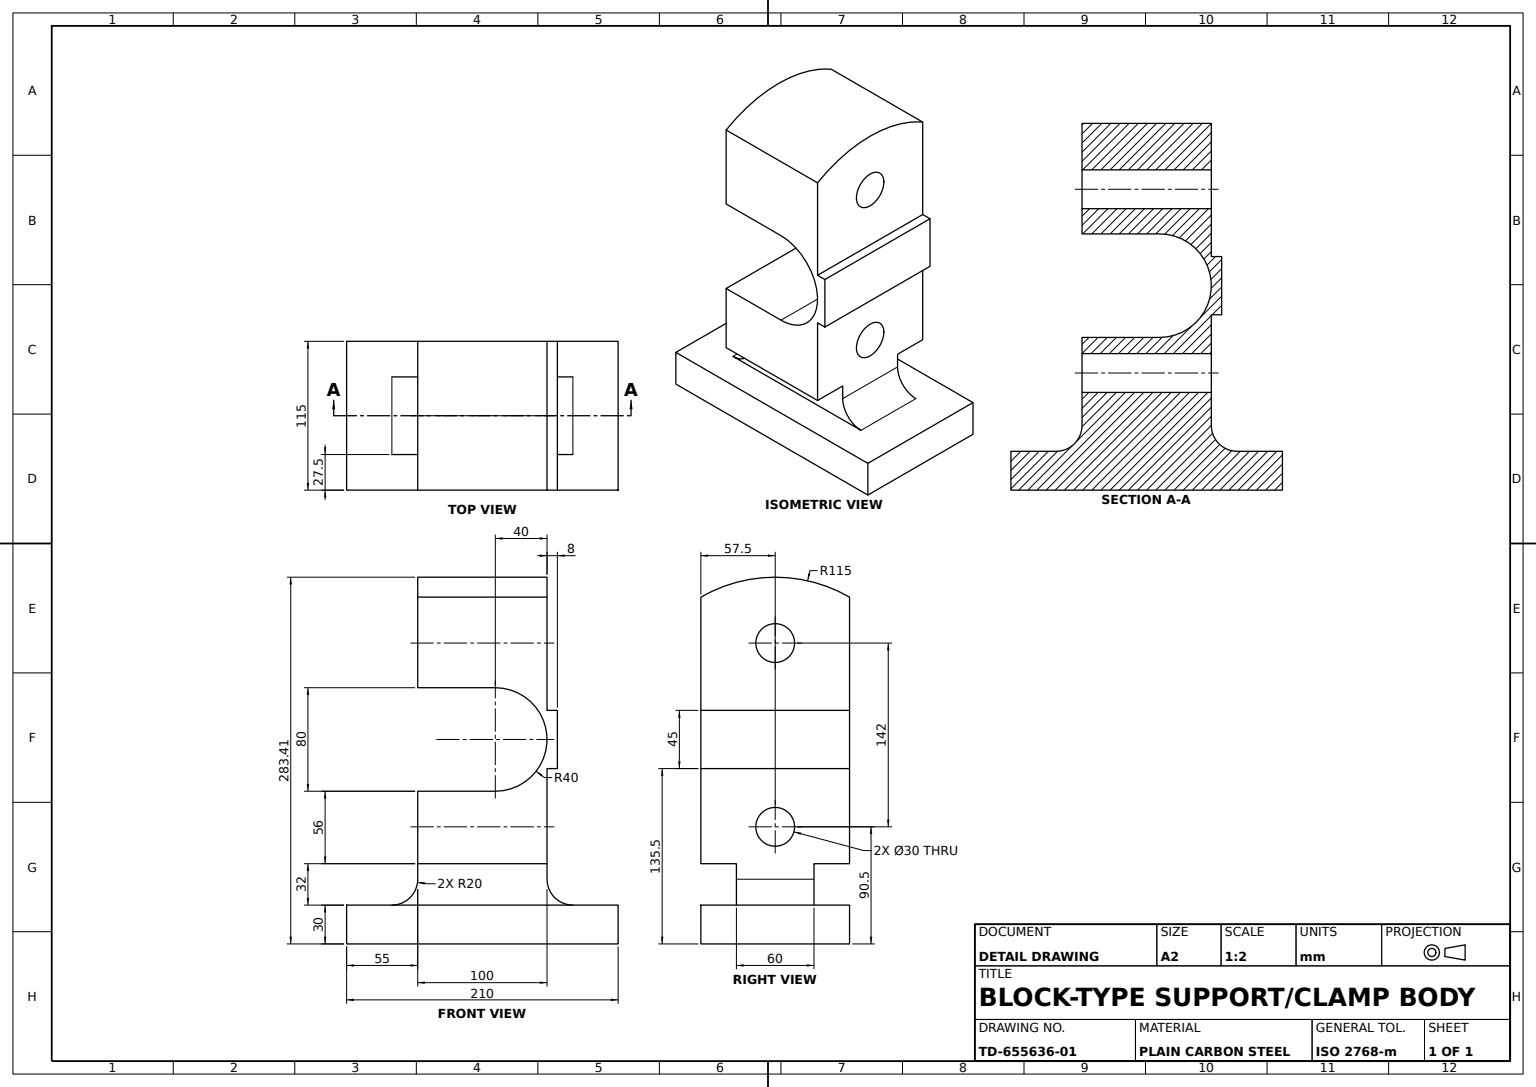
from build123d import *

# Parameters (mm, degrees)
BASE_PLATE_SKETCH_W         = 210
BASE_PLATE_SKETCH_H         = 115
BASE_PLATE_210X115X30_DEPTH = 30
PEDESTAL_SKETCH_W           = 100
PEDESTAL_SKETCH_H           = 60
PEDESTAL_100X60X32_DEPTH    = 32
PEDESTAL_FILLET_R20_R       = 20
CLAMP_BLOCK_DEPTH           = 57.5
CROSS_HOLES_SKETCH_R        = 15
CROSS_HOLES_2X_30_DEPTH     = 115
CLAMP_BAND_DEPTH            = 100


with BuildPart() as part:
    # Base Plate Sketch → Base Plate 210x115x30 (new body)
    with BuildSketch(Plane(origin=(0, 0, 0), x_dir=(1, 0, 0), z_dir=(0, 1, 0))):
        Rectangle(BASE_PLATE_SKETCH_W, BASE_PLATE_SKETCH_H)
    extrude(amount=BASE_PLATE_210X115X30_DEPTH)

    # Pedestal Sketch → Pedestal 100x60x32 (add)
    with BuildSketch(Plane(origin=(0, 30, 0), x_dir=(1, 0, 0), z_dir=(0, 1, 0))):
        Rectangle(PEDESTAL_SKETCH_W, PEDESTAL_SKETCH_H)
    extrude(amount=PEDESTAL_100X60X32_DEPTH)

    # Pedestal Fillet R20
    pedestal_fillet_r20_edges = [part.edges().sort_by_distance(p)[0] for p in [
        (50, 30, 0),
        (-50, 30, 0),
    ]]
    fillet(pedestal_fillet_r20_edges, radius=PEDESTAL_FILLET_R20_R)

    # Clamp Block Profile Sketch → Clamp Block (add, symmetric)
    with BuildSketch(Plane.XY):
        with BuildLine():
            Line((50, 62), (50, 118))
            Line((50, 118), (50, 135.5))
            Line((50, 135.5), (58, 135.5))
            Line((58, 135.5), (58, 180.5))
            Line((58, 180.5), (50, 180.5))
            Line((50, 180.5), (50, 198))
            Line((50, 198), (50, 268))
            Line((50, 268), (-50, 268))
            Line((-50, 268), (-50, 198))
            Line((-50, 198), (10, 198))
            ThreePointArc((10, 198), (50, 158), (10, 118))
            Line((10, 118), (-50, 118))
            Line((-50, 118), (-50, 62))
            Line((-50, 62), (50, 62))
        make_face()
    extrude(amount=CLAMP_BLOCK_DEPTH, both=True)

    # Cross Holes Sketch → Cross Holes 2xØ30 (cut)
    with BuildSketch(Plane.ZY.offset(50)):
        with Locations((0, 90.5)):
            Circle(CROSS_HOLES_SKETCH_R)
        with Locations((0, 232.5)):
            Circle(CROSS_HOLES_SKETCH_R)
    extrude(amount=-CROSS_HOLES_2X_30_DEPTH, mode=Mode.SUBTRACT)

    # Clamp Band Sketch → Clamp Band (add)
    with BuildSketch(Plane.ZY.offset(50)):
        with BuildLine():
            Line((-57.5, 268), (57.5, 268))
            ThreePointArc((57.5, 268), (0, 283.407078565), (-57.5, 268))
        make_face()
    extrude(amount=-CLAMP_BAND_DEPTH)


solid = part.part
